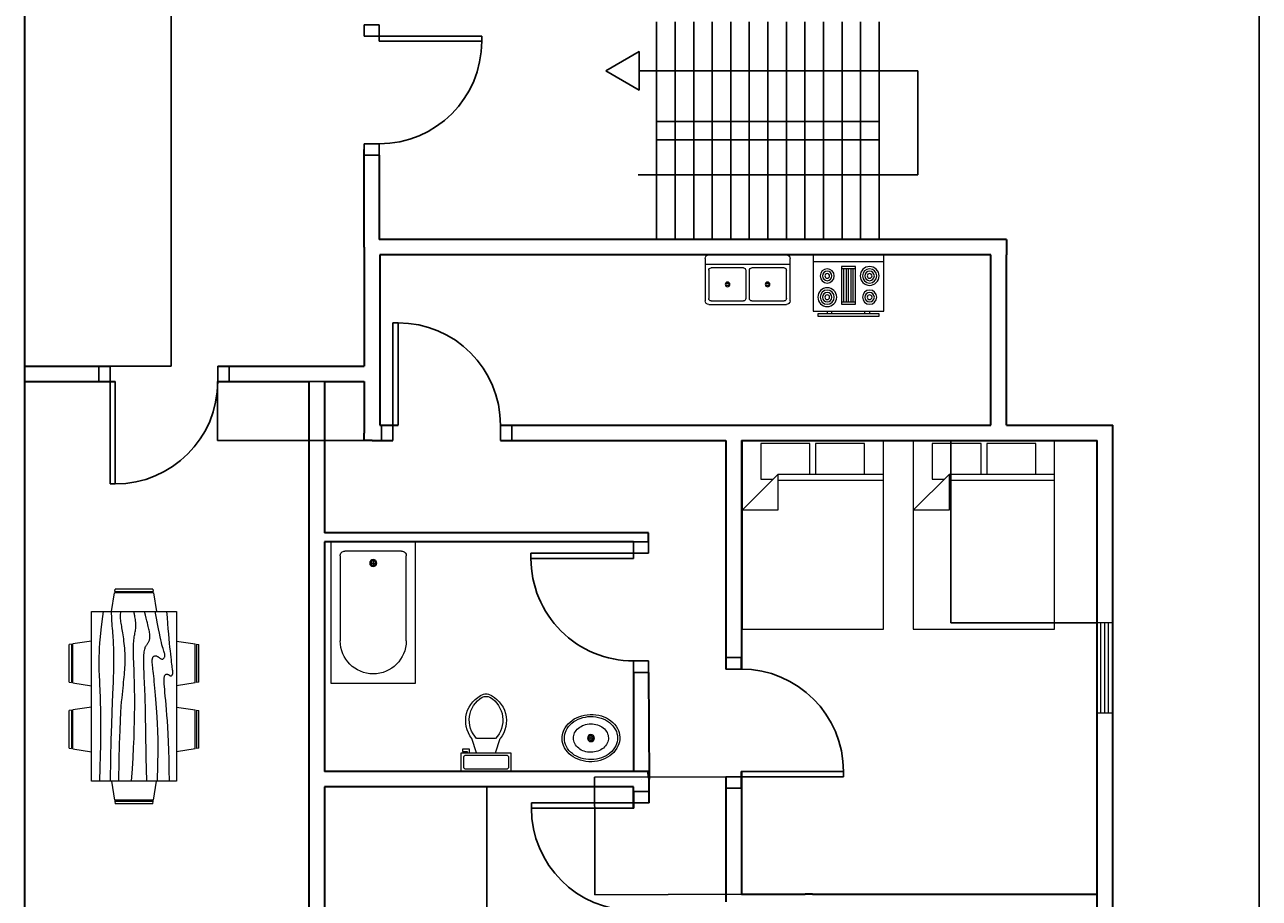
# Model space of a CAD drawing. Units: millimetres. Extents: x 31 to 27050, y -916 to 32407.
# Tile 4 of 7: x 13741 to 27050, y 7370 to 16782. Entities that reach past the tile are written whole.
import ezdxf

# ---------------------------------------------------------------- set-up
doc = ezdxf.new("R2010")
doc.units = ezdxf.units.MM
for name, color, linetype, lineweight in [('A-ANNO-DIMS', 2, 'Continuous', 18), ('A-DOOR', 3, 'Continuous', 25), ('A-EQPM', 8, 'Continuous', 18), ('A-FLOR-FIXT', 9, 'Continuous', 18), ('A-FLOR-STRS', 7, 'Continuous', 25), ('A-FURN', 8, 'Continuous', 13), ('A-GLAZ', 4, 'Continuous', 18), ('A-WALL', 7, 'Continuous', 35)]:
    doc.layers.add(name, color=color, linetype=linetype, lineweight=lineweight)
doc.styles.get("Standard").update_dxf_attribs({"font": 'arial.ttf'})
doc.dimstyles.get("Standard").update_dxf_attribs({"dimtxt": 0.18, "dimasz": 0.18, "dimexe": 0.18, "dimexo": 0.0625, "dimgap": 0.09, "dimtad": 0, "dimtih": 1, "dimtoh": 1, "dimdec": 4, "dimzin": 0, "dimdsep": 46, "dimtxsty": 'Standard', "dimcen": 0.09, "dimadec": 0, "dimazin": 0, "dimtfac": 1, "dimtdec": 4, "dimtofl": 0, "dimtmove": 0, "dimatfit": 3, "dimfxl": 1, "dimtolj": 1, "dimtzin": 0, "dimarcsym": 0})

# ---------------------------------------------------------------- blocks, each defined once
blk = doc.blocks.new('Bath Tub - 26 x 60 in.')
for p, q in [((8, -18), (10, -18)), ((9, -17), (9, -19))]:
    blk.add_line(p, q)
blk.add_lwpolyline([(0, -36), (0, 0), (60, 0), (60, -36)], close=True)
for points in [[(6, -4), (42, -4)], [(4, -30), (4, -6)], [(42, -32), (6, -32)]]:
    blk.add_lwpolyline(points)
for radius in [1.5, 1]:
    blk.add_circle((9, -18), radius)
for centre, radius, start, end in [((5.75, -5.75), 1.767766999999999, 81.86989999999999, 188.1301), ((42, -18), 14, 270, 90), ((5.75, -30.25), 1.767766999999999, 171.8699, 278.1301)]:
    blk.add_arc(centre, radius, start, end)
blk = doc.blocks.new('Sink - Oval top')
for p, q in [((-1, 0), (1, 0)), ((0, 1), (0, -1))]:
    blk.add_line(p, q)
for points in [[(-12.23371880354079, 0.3941914712607968, 0.1176342565883263), (-11.46456229543957, -3.361933235489118, 0.104469279667093), (-8.878748691070427, -6.803541973650567, 0.0900157896014849), (-5.082757700676665, -9.072309807490512, 0.0819199491592185), (-0.3227280122732736, -10.01585280257211, 0.0819199491592091), (4.488169920880977, -9.380701564817912, 0.0900157896014801), (8.422342359155778, -7.36101289847943, 0.1044692796670922), (11.22435122606941, -4.093009071543406, 0.1176342565883338), (12.23371880354091, -0.3941914712607968, 0.1176342565883057), (11.46456229543992, 3.361933235488777, 0.1044692796670849), (8.878748691070427, 6.803541973650567, 0.0900157896014884), (5.082757700676324, 9.072309807490681, 0.0819199491592058), (0.3227280122732736, 10.01585280257211, 0.081919949159207), (-4.488169920880864, 9.380701564817969, 0.0900157896014802), (-8.422342359155778, 7.36101289847943, 0.1044692796670951), (-11.22435122606919, 4.093009071543633, 0.1176342565883402)], [(-11.28627986850119, 0.1590597164737346, 0.1186217001864142), (-10.51590095791209, -3.253161772358112, 0.1046781721811095), (-8.071803350560115, -6.358618019863342, 0.0895620664691738), (-4.537699193222351, -8.366971929609804, 0.0811846988912177), (-0.1289739026695997, -9.15150355811437, 0.0811846988912276), (4.300109150126218, -8.491524865184601, 0.0895620664691798), (7.889406708212618, -6.583562428127606, 0.1046781721811044), (10.42004782883111, -3.548216131892445, 0.1186217001864013), (11.28627986850119, -0.1590597164736209, 0.1186217001863945), (10.51590095791221, 3.253161772357998, 0.1046781721811069), (8.071803350560115, 6.358618019863342, 0.0895620664691756), (4.537699193222124, 8.366971929609917, 0.081184698891216), (0.1289739026695997, 9.151503558114428, 0.0811846988912142), (-4.300109150125877, 8.491524865184829, 0.0895620664691747), (-7.889406708212618, 6.583562428127606, 0.1046781721811045), (-10.42004782883111, 3.548216131892445, 0.1186217001863946)], [(-7.420452389032902, 0.0829876781601797, 0.1182825673856775), (-6.907065465214486, -2.1674649380775, 0.1046074595377274), (-5.294791470712084, -4.209988192029413, 0.0897179636260996), (-2.966599981142508, -5.528122152688069, 0.0814360825277113), (-0.0675135187855176, -6.036810076758797, 0.0814360825277218), (2.84222437824053, -5.593085960977873, 0.0897179636261315), (5.199312936802016, -4.327350491993342, 0.1046074595376878), (6.85686365682659, -2.321395784920355, 0.1182825673856714), (7.420452389033016, -0.0829876781601797, 0.1182825673856961), (6.907065465214486, 2.167464938077614, 0.1046074595377135), (5.294791470712084, 4.209988192029413, 0.0897179636261265), (2.966599981142621, 5.528122152687842, 0.0814360825277426), (0.0675135187855176, 6.036810076758797, 0.0814360825277225), (-2.842224378240644, 5.593085960977873, 0.0897179636261212), (-5.199312936802016, 4.327350491993342, 0.1046074595377049), (-6.856863656826476, 2.321395784920355, 0.1182825673856712)]]:
    blk.add_lwpolyline(points, format="xyb", close=True)
for radius in [1.5, 1]:
    blk.add_circle((0, 0), radius)
blk = doc.blocks.new('Toilet - top')
for p, q in [((9.5, -6), (9.5, -2)), ((-10, -8.5), (-8, -8.5)), ((-10, -9.5), (-10, -8.5)), ((-7, -9.5), (-10, -9.5)), ((-8, -8.5), (-8, -8)), ((-7, -8), (-7, -9.5)), ((-4, -8), (-6, -14)), ((4, -8), (6, -14)), ((4, -14), (-4, -14))]:
    blk.add_line(p, q)
blk.add_lwpolyline([(10.5, -8), (10.5, 0), (-10.5, 0), (-10.5, -8)], close=True)
for points in [[(-9.5, -2), (-9.5, -6)], [(8.5, -1), (-8.5, -1)], [(-8.5, -7), (8.5, -7)]]:
    blk.add_lwpolyline(points)
for centre, radius, start, end in [((-8.625, -1.875), 0.8838834999999999, 81.86989999999999, 188.1301), ((8.625, -1.875), 0.8838834999999999, 351.8699, 98.13009999999998), ((-8.625, -6.125), 0.8838834999999999, 171.869898, 278.1301), ((8.625, -6.125), 0.8838834999999999, 261.8699, 8.130099999999993), ((3.519562435188956, -21.58049502388982), 12.16902005083646, 141.4691096810948, 247.9714346835576), ((4.199957580658807, -21.81740929088453), 11.3291791325804, 136.3677254423718, 238.946823937405), ((-3.519499936778316, -21.58047137067522), 12.16903423757823, 292.0284332733152, 38.53070636800453), ((-4.199890672038477, -21.81738596564128), 11.32918622148567, 301.0530065773863, 43.63209216694732), ((2.09660981727e-05, -27.87646475467881), 4, 245.7318247449371, 294.2681740488959), ((2.09415214183e-05, -28.99996806116075), 4, 254.8605283244437, 285.1394707718433)]:
    blk.add_arc(centre, radius, start, end)
blk = doc.blocks.new('Dining Set - 36 x 72 in.')
for p, q in [((-22, 27.5), (-22.15620000000001, 26.50042)), ((-5.841600000000028, 26.5), (-22.15340000000003, 26.5)), ((-22, 27.5), (-6, 27.5)), ((-5.843700000000012, 26.49966), (-6, 27.5)), ((6, 27.5), (5.843799999999987, 26.50042)), ((22.15839999999997, 26.5), (5.846599999999966, 26.5)), ((6, 27.5), (22, 27.5)), ((22.15629999999999, 26.49966), (22, 27.5)), ((-22.23430000000002, 26.00059), (-23.48470000000003, 17.99762)), ((-22.23040000000003, 26), (-5.760800000000017, 26)), ((-4.515199999999992, 17.99762), (-5.765500000000031, 25.99926)), ((5.765699999999981, 26.00059), (4.515299999999967, 17.99762)), ((5.769599999999968, 26), (22.23919999999998, 26)), ((23.48480000000001, 17.99762), (22.23449999999997, 25.99926)), ((36, 18), (-36, 18)), ((-36, 18), (-36, -18)), ((36, -18), (36, 18)), ((-45.49999999999999, 8.000000000000004), (-44.50040000000001, 8.156170000000007)), ((-45.49999999999999, 8.000000000000004), (-45.49999999999999, -7.999999999999996)), ((-44.5, -8.15843), (-44.5, 8.153380000000002)), ((-44.00060000000002, 8.234280000000002), (-35.99760000000003, 9.484740000000006)), ((-44, 8.230410000000003), (-44, -8.239149999999999)), ((44.00059999999996, 8.234280000000002), (35.99759999999998, 9.484740000000006)), ((44, 8.230410000000003), (44, -8.239149999999999)), ((44.5, -8.15843), (44.5, 8.153380000000002)), ((45.49999999999999, 8.000000000000004), (44.50049999999999, 8.156170000000007)), ((45.49999999999999, 8.000000000000004), (45.49999999999999, -7.999999999999996)), ((-44.49970000000002, -8.156309999999994), (-45.49999999999999, -7.999999999999996)), ((-35.99760000000003, -9.484759999999998), (-43.9993, -8.234499999999993)), ((35.99759999999998, -9.484759999999998), (43.9993, -8.234499999999993)), ((44.49969999999995, -8.156309999999994), (45.49999999999999, -7.999999999999996)), ((-36, -18), (36, -18)), ((-22.23430000000002, -26.0006), (-23.48470000000003, -17.99762)), ((-4.515199999999992, -17.99762), (-5.765500000000031, -25.99928)), ((5.765699999999981, -26.0006), (4.515299999999967, -17.99762)), ((23.48480000000001, -17.99762), (22.23449999999997, -25.99928)), ((-22.23040000000003, -26), (-5.760800000000017, -26)), ((5.769599999999968, -26), (22.23919999999998, -26)), ((-22, -27.5), (-22.15620000000001, -26.50044)), ((-5.841600000000028, -26.5), (-22.15340000000003, -26.5)), ((-22, -27.5), (-6, -27.5)), ((-5.843700000000012, -26.49967), (-6, -27.5)), ((6, -27.5), (5.843799999999987, -26.50044)), ((22.15839999999997, -26.5), (5.846599999999966, -26.5)), ((6, -27.5), (22, -27.5)), ((22.15629999999999, -26.49967), (22, -27.5))]:
    blk.add_line(p, q)
for points in [[(-36, 15), (-31.17720000000003, 14.97754), (-26.80790000000002, 14.91406), (-22.85380000000003, 14.81543), (-19.27600000000001, 14.6875), (-16.03620000000001, 14.53613), (-13.09570000000002, 14.36718), (-10.41590000000002, 14.18652), (-7.958300000000008, 14), (-5.690400000000011, 13.81315), (-3.603499999999996, 13.63021), (-1.695400000000006, 13.45508), (0.0364999999999896, 13.29166), (1.594499999999982, 13.14388), (2.981099999999969, 13.01562), (4.198800000000005, 12.9108), (5.25, 12.83333), (6.139299999999991, 12.78613), (6.880200000000002, 12.76823), (7.488299999999981, 12.77767), (7.979199999999991, 12.8125), (8.368499999999983, 12.87077), (8.671899999999994, 12.95052), (8.904899999999998, 13.0498), (9.083300000000008, 13.16666), (9.220499999999959, 13.29899000000001), (9.32159999999999, 13.44401), (9.389499999999998, 13.59879), (9.427099999999996, 13.76041), (9.437299999999993, 13.92594), (9.423200000000008, 14.09245), (9.387499999999989, 14.257), (9.333300000000008, 14.41666), (9.263800000000003, 14.56917), (9.183600000000013, 14.71484), (9.097499999999968, 14.85465), (9.010400000000004, 14.98958), (8.92719999999997, 15.12060000000001), (8.852899999999975, 15.2487), (8.79219999999998, 15.37483), (8.75, 15.5), (8.730500000000006, 15.62467), (8.734399999999994, 15.74739), (8.761699999999962, 15.86621), (8.8125, 15.97916), (8.886699999999962, 16.08431), (8.984399999999994, 16.17968), (9.105500000000006, 16.26334), (9.25, 16.33333), (9.418900000000008, 16.38802), (9.617199999999968, 16.42708), (9.850599999999986, 16.45052), (10.125, 16.45833), (10.44630000000001, 16.45052), (10.82029999999997, 16.42708), (11.25290000000001, 16.38802), (11.75, 16.33333), (12.3184, 16.26318), (12.96940000000001, 16.17838), (13.7151, 16.07991), (14.5677, 15.96875), (15.53949999999997, 15.84586), (16.64259999999996, 15.71224), (17.88929999999999, 15.56884), (19.29169999999999, 15.41666), (20.85899999999998, 15.25667), (22.58789999999999, 15.08984), (24.47210000000001, 14.91715), (26.5052, 14.73958), (28.68090000000001, 14.5581), (30.99289999999996, 14.3737), (33.43469999999996, 14.18733), (36, 14)], [(-36, 10), (-28.97660000000002, 10.14274000000001), (-23.17250000000001, 10.20442), (-18.42410000000001, 10.19775), (-14.5677, 10.13541), (-11.43990000000002, 10.03011), (-8.87700000000001, 9.894530000000007), (-6.715399999999988, 9.741370000000005), (-4.791699999999991, 9.58333), (-2.96980000000002, 9.43082), (-1.224600000000009, 9.285150000000005), (0.4414999999999623, 9.14534), (2.02600000000001, 9.010410000000004), (3.526599999999973, 8.879390000000004), (4.940799999999967, 8.751300000000004), (6.265999999999962, 8.625160000000005), (7.5, 8.500000000000004), (8.641099999999994, 8.375490000000003), (9.691399999999987, 8.253900000000005), (10.65379999999999, 8.13818), (11.53120000000001, 8.031250000000004), (12.32669999999996, 7.936030000000005), (13.043, 7.85547), (13.68309999999997, 7.792480000000001), (14.25, 7.750000000000003), (14.74709999999999, 7.730300000000003), (15.17969999999997, 7.733070000000001), (15.55369999999999, 7.757320000000003), (15.875, 7.80208), (16.14940000000001, 7.866370000000006), (16.38279999999997, 7.94922), (16.58109999999999, 8.04964), (16.75, 8.166660000000004), (16.89439999999996, 8.29915), (17.01429999999999, 8.445310000000003), (17.1089, 8.603190000000001), (17.17709999999999, 8.77083), (17.21799999999996, 8.946290000000001), (17.2305, 9.127600000000005), (17.21369999999996, 9.312820000000006), (17.16669999999999, 9.500000000000004), (17.08949999999999, 9.687500000000004), (16.98699999999996, 9.875000000000004), (16.86489999999998, 10.0625), (16.72919999999999, 10.25), (16.5856, 10.4375), (16.44009999999997, 10.625), (16.29849999999999, 10.8125), (16.16669999999999, 11), (16.05000000000001, 11.18733), (15.95179999999999, 11.3737), (15.8752, 11.5581), (15.8229, 11.73958), (15.798, 11.91715), (15.80340000000001, 12.08984), (15.84199999999998, 12.25667), (15.91669999999999, 12.41666), (16.02949999999998, 12.56836), (16.17840000000001, 12.70833), (16.3605, 12.83268), (16.5729, 12.9375), (16.8127, 13.01888000000001), (17.07679999999999, 13.07291), (17.36250000000001, 13.0957), (17.66669999999999, 13.08333), (17.98939999999999, 13.03312), (18.34179999999998, 12.94726), (18.7382, 12.82918), (19.1927, 12.68229), (19.71949999999998, 12.51001), (20.33269999999999, 12.31575), (21.04649999999998, 12.10294), (21.875, 11.875), (22.83569999999997, 11.63354), (23.95900000000001, 11.37304), (25.27859999999999, 11.08618), (26.82819999999998, 10.76562), (28.64139999999998, 10.40405), (30.75200000000001, 9.994140000000005), (33.1936, 9.528560000000002), (36, 9.000000000000004)], [(-36, 5.500000000000003), (-30.71570000000003, 5.334800000000004), (-26.06900000000002, 5.20963), (-21.99459999999999, 5.11767), (-18.42709999999999, 5.05208), (-15.30090000000001, 5.006020000000003), (-12.55080000000004, 4.972650000000005), (-10.1112, 4.945150000000001), (-7.916699999999991, 4.916660000000003), (-5.908999999999991, 4.881670000000003), (-4.058600000000012, 4.839840000000005), (-2.342899999999985, 4.792150000000003), (-0.7395999999999959, 4.73958), (0.7738999999999692, 4.683100000000006), (2.21999999999997, 4.623700000000003), (3.621299999999962, 4.562330000000006), (5, 4.500000000000003), (6.37299999999999, 4.437820000000005), (7.734399999999993, 4.377600000000004), (9.072299999999984, 4.321290000000001), (10.375, 4.27083), (11.63089999999999, 4.228190000000001), (12.8281, 4.195310000000002), (13.95509999999996, 4.17415), (15, 4.166660000000003), (15.95400000000001, 4.174480000000006), (16.81899999999996, 4.197910000000003), (17.6001, 4.236980000000006), (18.30209999999999, 4.291660000000003), (18.92989999999997, 4.361980000000006), (19.48829999999998, 4.447910000000003), (19.98230000000001, 4.549480000000006), (20.41669999999999, 4.666660000000003), (20.79689999999999, 4.798990000000006), (21.1302, 4.944010000000002), (21.42449999999997, 5.098790000000004), (21.6875, 5.260410000000003), (21.92709999999999, 5.42594), (22.15109999999999, 5.592450000000003), (22.36719999999997, 5.757000000000001), (22.58339999999998, 5.916660000000003), (22.80649999999997, 6.068680000000004), (23.04039999999998, 6.210930000000001), (23.28789999999998, 6.341470000000004), (23.5521, 6.45833), (23.83580000000001, 6.559570000000004), (24.142, 6.643230000000006), (24.4735, 6.707350000000001), (24.83339999999998, 6.750000000000003), (25.2235, 6.76969), (25.642, 6.766920000000002), (26.08580000000001, 6.74267), (26.5521, 6.697910000000003), (27.03789999999998, 6.633620000000004), (27.54039999999998, 6.550780000000006), (28.05649999999997, 6.450360000000006), (28.58339999999998, 6.33333), (29.12419999999997, 6.19987), (29.70709999999997, 6.046870000000001), (30.36609999999996, 5.870440000000005), (31.1354, 5.666660000000003), (32.04929999999996, 5.431640000000005), (33.142, 5.161460000000001), (34.44749999999999, 4.852210000000003), (36, 4.500000000000003)], [(-36, -0.9999999999999964), (-30.79150000000004, -0.6590999999999987), (-26.01949999999999, -0.3821599999999954), (-21.65190000000001, -0.1628399999999992), (-17.65629999999999, 0.0052100000000017), (-14.00049999999999, 0.1283300000000018), (-10.65230000000002, 0.2128900000000051), (-7.579600000000027, 0.2652200000000029), (-4.75, 0.2916600000000038), (-2.134000000000014, 0.2979300000000045), (0.2878000000000043, 0.287110000000002), (2.5317, 0.2616300000000002), (4.614599999999995, 0.2239600000000017), (6.552899999999965, 0.1765100000000039), (8.363299999999981, 0.1217400000000062), (10.06229999999999, 0.0620900000000013), (11.66669999999999, 3.6e-15), (13.18989999999996, -0.0620099999999972), (14.63409999999999, -0.1210999999999949), (15.9982, -0.174319999999998), (17.28129999999999, -0.2187499999999964), (18.48230000000001, -0.2514699999999941), (19.6003, -0.2695299999999996), (20.6343, -0.2700199999999988), (21.58339999999999, -0.2499999999999964), (22.44810000000001, -0.2076799999999999), (23.23570000000001, -0.1458399999999962), (23.95490000000001, -0.0683599999999949), (24.6146, 0.0208300000000001), (25.2235, 0.1178400000000046), (25.79039999999998, 0.2187500000000035), (26.32409999999999, 0.3196600000000025), (26.83339999999998, 0.4166600000000038), (27.32650000000001, 0.5061800000000041), (27.80989999999997, 0.5859300000000012), (28.2894, 0.6539700000000046), (28.77089999999999, 0.7083300000000002), (29.26009999999997, 0.7470700000000045), (29.76299999999998, 0.7682300000000062), (30.28550000000001, 0.7698500000000017), (30.83339999999998, 0.7500000000000036), (31.40879999999999, 0.707840000000001), (31.99939999999998, 0.6471300000000006), (32.589, 0.5727500000000028), (33.16149999999999, 0.4895800000000002), (33.70079999999996, 0.402500000000007), (34.19079999999997, 0.3164000000000051), (34.61529999999999, 0.2361600000000017), (34.95839999999998, 0.1666600000000038), (35.20990000000001, 0.1116500000000009), (35.38479999999998, 0.0703100000000028), (35.50399999999996, 0.0406900000000015), (35.58859999999999, 0.0208300000000001), (35.65940000000001, 0.0087900000000012), (35.73769999999996, 0.0026000000000046), (35.8442, 0.0003200000000056), (36, 3.6e-15)], [(-36, -6.499999999999996), (-27.18430000000001, -6.312669999999993), (-20.084, -6.126299999999996), (-14.46899999999999, -5.941899999999993), (-10.10939999999999, -5.760419999999999), (-6.77520000000004, -5.582849999999996), (-4.236300000000028, -5.410159999999994), (-2.262900000000001, -5.243329999999996), (-0.625, -5.083339999999996), (0.8707999999999742, -4.930989999999997), (2.271500000000003, -4.786459999999994), (3.587199999999995, -4.649739999999997), (4.828100000000006, -4.520839999999996), (6.004599999999982, -4.399739999999997), (7.127000000000009, -4.286459999999994), (8.205299999999966, -4.180989999999997), (9.25, -4.083339999999996), (10.27049999999997, -3.993819999999995), (11.27339999999998, -3.914069999999998), (12.2647, -3.846029999999995), (13.25, -3.791669999999999), (14.23539999999997, -3.752929999999995), (15.22659999999996, -3.731769999999993), (16.22949999999997, -3.730149999999998), (17.25, -3.749999999999996), (18.2912, -3.792479999999994), (19.3451, -3.855469999999993), (20.40089999999998, -3.936039999999994), (21.4479, -4.031249999999996), (22.47539999999998, -4.138189999999998), (23.47269999999998, -4.253909999999994), (24.4289, -4.375489999999995), (25.33339999999999, -4.499999999999996), (26.17849999999999, -4.624919999999999), (26.96940000000001, -4.749349999999996), (27.71449999999999, -4.872809999999997), (28.4219, -4.994789999999998), (29.09999999999996, -5.114829999999994), (29.75720000000001, -5.232419999999994), (30.40159999999997, -5.347089999999997), (31.04169999999999, -5.458339999999996), (31.68369999999999, -5.564369999999993), (32.32619999999997, -5.658209999999993), (32.9658, -5.731529999999995), (33.59899999999999, -5.776039999999998), (34.22239999999999, -5.783449999999998), (34.83269999999999, -5.745449999999994), (35.4264, -5.653729999999999), (36, -5.499999999999996)], [(-36, -9.999999999999996), (-26.40219999999999, -9.812989999999996), (-18.46750000000003, -9.628909999999994), (-11.9839, -9.450689999999998), (-6.739599999999995, -9.281249999999996), (-2.522600000000011, -9.123539999999995), (0.8788999999999872, -8.980469999999993), (3.676899999999989, -8.854979999999994), (6.083300000000008, -8.749999999999996), (8.276700000000005, -8.667649999999998), (10.30209999999999, -8.606769999999994), (12.1712, -8.565429999999996), (13.89580000000001, -8.54167), (15.48759999999998, -8.533529999999995), (16.95830000000001, -8.539069999999999), (18.31970000000001, -8.556319999999994), (19.58339999999998, -8.583339999999996), (20.76159999999999, -8.618409999999994), (21.86849999999998, -8.660809999999994), (22.91879999999998, -8.710039999999996), (23.9271, -8.765629999999998), (24.90809999999999, -8.827069999999996), (25.87629999999996, -8.89388), (26.84649999999999, -8.96558), (27.83339999999999, -9.04167), (28.84739999999999, -9.121179999999997), (29.88279999999998, -9.201169999999994), (30.93000000000001, -9.278239999999993), (31.97919999999999, -9.348959999999995), (33.02049999999997, -9.409909999999998), (34.04429999999996, -9.45768), (35.04069999999996, -9.488849999999996), (36, -9.499999999999996)], [(-36, -14.5), (-30.0881, -14.33512999999999), (-25.03320000000002, -14.21224), (-20.7312, -14.12646999999999), (-17.0781, -14.07292), (-13.97000000000003, -14.04670999999999), (-11.30270000000001, -14.04296999999999), (-8.972399999999993, -14.05680999999999), (-6.875, -14.08333999999999), (-4.922400000000038, -14.11832999999999), (-3.09050000000002, -14.16015999999999), (-1.370900000000006, -14.20784999999999), (0.2447999999999979, -14.26042), (1.764700000000004, -14.31689999999999), (3.197299999999984, -14.37629999999999), (4.550700000000006, -14.43766999999999), (5.833300000000008, -14.5), (7.055399999999963, -14.5621), (8.235000000000014, -14.62174999999999), (9.392200000000003, -14.67652), (10.54689999999999, -14.72395999999999), (11.7192, -14.76164), (12.92899999999997, -14.78711), (14.19649999999996, -14.79794), (15.54169999999999, -14.79167), (16.99329999999998, -14.76423999999999), (18.61519999999996, -14.70508), (20.48039999999998, -14.60197), (22.66149999999999, -14.44270999999999), (25.2312, -14.21509), (28.26240000000002, -13.90689999999999), (31.8277, -13.50594), (36, -13)]]:
    blk.add_lwpolyline(points)
blk = doc.blocks.new('Range-Oven - 30 in top')
for p, q in [((0, -3), (30, -3)), ((12, -6), (18, -6)), ((13, -19.999996), (13, -6)), ((14, -6), (14, -19.999996)), ((15, -19.999996), (15, -6)), ((16, -6), (16, -19.999996)), ((17, -19.999996), (17, -6)), ((18, -19.999996), (12, -19.999996)), ((6.000000000000003, -23.99999600000001), (6.000000000000003, -24.999996)), ((8.000000000000004, -24.999996), (8.000000000000004, -23.99999600000001)), ((22.00000000000001, -24.999996), (22.00000000000001, -23.99999600000001)), ((24, -23.99999600000001), (24, -24.999996))]:
    blk.add_line(p, q)
for points in [[(0, -23.99999600000001), (0, 0), (30, 0), (30, -23.99999600000001)], [(12, -20.999996), (12, -5), (18, -5), (18, -20.999996)], [(2.000000000000003, -25.999996), (2.000000000000003, -24.999996), (28.00000000000001, -24.999996), (28.00000000000001, -25.999996)]]:
    blk.add_lwpolyline(points, close=True)
for centre, radius in [((6.000000000000003, -9.0000002), 4), ((6.000000000000003, -9.0000002), 3), ((6.000000000000003, -9.0000002), 2), ((6.000000000000003, -9.0000002), 1), ((24, -9.0000002), 3), ((24, -9.0000002), 2), ((24, -9.0000002), 1), ((6.000000000000003, -18), 3), ((24, -18), 4), ((24, -18), 3), ((6.000000000000003, -18), 2), ((6.000000000000003, -18), 1), ((24, -18), 2), ((24, -18), 1)]:
    blk.add_circle(centre, radius)
blk = doc.blocks.new('Sink-double - 36 in top')
for p, q in [((-18, -4), (18, -4)), ((-0.75, -18.5), (-0.75, -6.5)), ((0.75, -6.5), (0.75, -18.5))]:
    blk.add_line(p, q)
for points in [[(-16.5, 0), (16.5, 0)], [(-18, -19.5), (-18, -1.5)], [(18, -1.5), (18, -19.5)], [(-16.5, -18.5), (-16.5, -6.5)], [(-15.5, -5.5), (-1.75, -5.5)], [(1.75, -5.5), (15.5, -5.5)], [(16.5, -6.5), (16.5, -18.5)], [(-1.75, -19.5), (-15.5, -19.5)], [(15.5, -19.5), (1.75, -19.5)], [(16.5, -21), (-16.5, -21)]]:
    blk.add_lwpolyline(points)
for centre, radius in [((-8.5, -12.5), 1), ((-8.5, -12.5), 0.5), ((8.5, -12.5), 1), ((8.5, -12.5), 0.5)]:
    blk.add_circle(centre, radius)
for centre, radius, start, end in [((-16.5, -1.5), 1.5, 90, 180), ((16.5, -1.5), 1.5, 0, 90), ((-15.5, -6.5), 1, 90, 180), ((-1.75, -6.5), 1, 0, 90), ((1.75, -6.5), 1, 90, 180), ((15.5, -6.5), 1, 0, 90), ((-16.5, -19.5), 1.5, 180, 270), ((-15.5, -18.5), 1, 180, 270), ((-1.75, -18.5), 1, 270, 0), ((1.75, -18.5), 1, 180, 270), ((15.5, -18.5), 1, 270, 0), ((16.5, -19.5), 1.5, 270, 0)]:
    blk.add_arc(centre, radius, start, end)
blk = doc.blocks.new('Bed - Queen')
for p, q in [((0, -80.00003000000002), (0, 0)), ((0, 0), (59.99998999999999, 0)), ((59.99998999999999, 0), (59.99998999999999, -80.00003000000002)), ((7.99999, -1.200000000000017), (28.79998, -1.200000000000017)), ((7.99999, -14.4), (7.99999, -1.200000000000017)), ((28.79998, -1.200000000000017), (28.79998, -14.4)), ((31.19999, -1.200000000000017), (51.99999000000001, -1.200000000000017)), ((31.19999, -14.4), (31.19999, -1.200000000000017)), ((51.99999000000001, -1.200000000000017), (51.99999000000001, -16.4)), ((0, -14.4), (44.79999999999999, -14.4)), ((59.99998999999999, -29.60000000000001), (44.79999999999999, -14.4)), ((44.79999999999999, -14.4), (44.79999999999999, -29.60000000000001)), ((44.79999999999999, -16.80000000000001), (0, -16.80000000000001)), ((51.99999000000001, -16.4), (46.79936, -16.4)), ((44.79999999999999, -29.60000000000001), (59.99998999999999, -29.60000000000001)), ((59.99998999999999, -80.00003000000002), (0, -80.00003000000002))]:
    blk.add_line(p, q)
blk = doc.blocks.new('Window - Wood Frame 36 in. Wide plan')
for p, q in [((0, 6), (0, 0)), ((36, 6), (36, 0)), ((0, 4.5), (36, 4.5)), ((0, 3), (36, 3)), ((0, 1.5), (36, 1.5))]:
    blk.add_line(p, q)
blk = doc.blocks.new('DOOR-SINGLE-1104')
for p, q in [((56.41678681898429, 1104.337341461596), (-7.18501e-11, 1104.337341461596)), ((-7.18501e-11, 1104.337341461596), (-7.18501e-11, 3.638e-12)), ((56.41678681898429, 7.276e-12), (56.41678681898429, 1104.337341461596)), ((-1226.913698425656, -163.8831223050438), (-1226.913698425656, 3.638e-12)), ((-1104.337341461589, 3.638e-12), (-1226.913698425656, 7.276e-12)), ((-1104.337341461589, 3.638e-12), (-1104.337341461589, -163.8831223050438)), ((-7.18501e-11, 3.638e-12), (56.41678681898429, 7.276e-12)), ((56.41678681898429, -163.8831223050438), (56.41678681898429, 3.638e-12)), ((56.41678681898429, 3.638e-12), (178.9931437830519, 3.638e-12)), ((178.9931437830519, 3.638e-12), (178.9931437830519, -163.8831223050438)), ((-1104.337341461589, -163.8831223050438), (-1226.913698425656, -163.8831223050438)), ((178.9931437830519, -163.8831223050438), (56.41678681898429, -163.8831223050438))]:
    blk.add_line(p, q)
blk.add_arc((0, 3.638e-12), 1104.337341461589, 90, 180)
blk = doc.blocks.new('STAIR-RETURN-2400')
for p, q in [((9.095e-13, 2345.636859649549), (9.095e-13, -1.819e-12)), ((200.0000000000009, 2345.636859649549), (200.0000000000009, -1.819e-12)), ((400.0000000000008, 2345.636859649549), (400.0000000000008, -1.819e-12)), ((600.0000000000008, 2345.636859649549), (600.0000000000008, -1.819e-12)), ((800.0000000000008, 2345.636859649552), (800.0000000000008, 1.819e-12)), ((1000.000000000001, 2345.636859649556), (1000.000000000001, 5.457e-12)), ((1200.000000000001, 2345.636859649556), (1200.000000000001, 5.457e-12)), ((1400.000000000001, 2345.636859649556), (1400.000000000001, 5.457e-12)), ((1600.000000000001, 2345.636859649559), (1600.000000000001, 9.0949e-12)), ((1800.000000000001, 2345.636859649559), (1800.000000000001, 9.0949e-12)), ((2000.000000000001, 2345.636859649559), (2000.000000000001, 9.0949e-12)), ((2200.000000000001, 2345.636859649563), (2200.000000000001, 1.27329e-11)), ((2400.000000000001, 2345.636859649563), (2400.000000000001, 1.27329e-11)), ((-415.9249645337103, 697.4958917418807), (-415.9249645337103, 1817.654410237617)), ((-415.9249645337103, 1817.654410237617), (2588.331988211024, 1817.654410237617)), ((9.095e-13, 1172.818429824772), (9.095e-13, 1272.818429824772)), ((9.095e-13, 1272.818429824772), (2400.000000000001, 1272.818429824774)), ((2400.000000000001, 1272.818429824774), (2400.000000000001, 1072.818429824774)), ((2400.000000000001, 1072.818429824774), (9.095e-13, 1072.818429824774)), ((2597.09055342863, 697.4958917418807), (-415.9249645337103, 697.4958917418807))]:
    blk.add_line(p, q)
blk.add_lwpolyline([(2948.607295106225, 1817.654410237617), (2588.331988211024, 2025.65945565594), (2588.331988211024, 1609.649364819299)], close=True)
blk = doc.blocks.new('*D47')
at = {"layer": 'A-ANNO-DIMS', "color": 0, "lineweight": -2, "transparency": 16777216}
for p, q in [((25471.21116800002, 30827.53125900001), (27050.32866800003, 30827.53125900001)), ((27050.14866800003, 30827.35125900001), (27050.14866800003, 15745.77166202933)), ((27050.14866800004, 663.8281360000004), (27050.14866800003, 15745.40773297067)), ((25471.21116800002, 663.6481360000002), (27050.32866800003, 663.6481360000004))]:
    blk.add_line(p, q, dxfattribs=at)
at = {"layer": 'A-ANNO-DIMS', "color": 0, "transparency": 16777216}
for points in [[(27050.11866800003, 30827.35125900001), (27050.17866800003, 30827.35125900001), (27050.14866800003, 30827.53125900001)], [(27050.11866800004, 663.8281360000004), (27050.17866800004, 663.8281360000004), (27050.14866800004, 663.6481360000004)]]:
    blk.add_solid(points, dxfattribs=at)
at = {"layer": 'Defpoints', "color": 0, "transparency": 16777216}
for p in [(25471.14866800002, 30827.53125900001), (27050.14866800003, 30827.53125900001), (25471.14866800002, 663.6481360000002)]:
    blk.add_point(p, dxfattribs=at)
at = {"layer": 'A-ANNO-DIMS', "color": 0, "transparency": 16777216, "insert": (27050.14866800003, 15745.58969749999), "char_height": 0.18, "attachment_point": 5}
blk.add_mtext('\\A1;30164', dxfattribs=at)
blk = doc.blocks.new('*D65')
at = {"layer": 'A-ANNO-DIMS', "color": 0, "lineweight": -2, "transparency": 16777216}
for p, q in [((20302.73551700001, 8571.211099000004), (18723.61801700001, 8571.211099000004)), ((18723.79801700001, 8571.031099000003), (18723.79801700001, 4699.551179000002)), ((18723.79801700001, 827.7112590000002), (18723.79801700001, 4699.191179000002)), ((20302.73551700001, 827.5312590000003), (18723.61801700001, 827.5312590000002))]:
    blk.add_line(p, q, dxfattribs=at)
at = {"layer": 'A-ANNO-DIMS', "color": 0, "transparency": 16777216}
for points in [[(18723.76801700001, 8571.031099000003), (18723.82801700001, 8571.031099000003), (18723.79801700001, 8571.211099000004)], [(18723.76801700001, 827.7112590000002), (18723.82801700001, 827.7112590000002), (18723.79801700001, 827.5312590000002)]]:
    blk.add_solid(points, dxfattribs=at)
at = {"layer": 'Defpoints', "color": 0, "transparency": 16777216}
for p in [(18723.79801700001, 8571.211099000004), (20302.79801700001, 8571.211099000004), (20302.79801700001, 827.5312590000003)]:
    blk.add_point(p, dxfattribs=at)
at = {"layer": 'A-ANNO-DIMS', "color": 0, "transparency": 16777216, "insert": (18723.79801700001, 4699.371178999996), "char_height": 0.18, "attachment_point": 5}
blk.add_mtext('\\A1;7744', dxfattribs=at)
blk = doc.blocks.new('*D67')
at = {"layer": 'A-ANNO-DIMS', "color": 0, "lineweight": -2, "transparency": 16777216}
for p, q in [((13740.64783300001, 17938.12750700001), (15319.76533300001, 17938.12750700001)), ((15319.58533300001, 17937.94750700001), (15319.58533300001, 15520.25103252934)), ((15319.58533300001, 13102.19062900001), (15319.58533300001, 15519.88710347067)), ((13740.64783300001, 13102.01062900001), (15319.76533300001, 13102.01062900001))]:
    blk.add_line(p, q, dxfattribs=at)
at = {"layer": 'A-ANNO-DIMS', "color": 0, "transparency": 16777216}
for points in [[(15319.55533300001, 17937.94750700001), (15319.61533300001, 17937.94750700001), (15319.58533300001, 17938.12750700001)], [(15319.55533300001, 13102.19062900001), (15319.61533300001, 13102.19062900001), (15319.58533300001, 13102.01062900001)]]:
    blk.add_solid(points, dxfattribs=at)
at = {"layer": 'Defpoints', "color": 0, "transparency": 16777216}
for p in [(13740.58533300001, 17938.12750700001), (13740.58533300001, 13102.01062900001), (15319.58533300001, 13102.01062900001)]:
    blk.add_point(p, dxfattribs=at)
at = {"layer": 'A-ANNO-DIMS', "color": 0, "transparency": 16777216, "insert": (15319.58533300002, 15520.069068), "char_height": 0.18, "attachment_point": 5}
blk.add_mtext('\\A1;4836', dxfattribs=at)
blk = doc.blocks.new('*D72')
at = {"layer": 'A-ANNO-DIMS', "color": 0, "lineweight": -2, "transparency": 16777216}
for p, q in [((17399.426108, 12938.12750700001), (15820.30860800001, 12938.12750700001)), ((15820.48860800001, 12937.947507), (15820.48860800001, 12620.17599252934)), ((15820.48860800001, 12302.04054900001), (15820.48860800001, 12619.81206347068)), ((17399.426108, 12301.860549), (15820.30860800001, 12301.860549))]:
    blk.add_line(p, q, dxfattribs=at)
at = {"layer": 'A-ANNO-DIMS', "color": 0, "transparency": 16777216}
for points in [[(15820.45860800001, 12937.947507), (15820.51860800001, 12937.947507), (15820.48860800001, 12938.12750700001)], [(15820.45860800001, 12302.04054900001), (15820.51860800001, 12302.04054900001), (15820.48860800001, 12301.860549)]]:
    blk.add_solid(points, dxfattribs=at)
at = {"layer": 'Defpoints', "color": 0, "transparency": 16777216}
for p in [(15820.48860800001, 12938.12750700001), (17399.48860800001, 12938.12750700001), (17399.48860800001, 12301.860549)]:
    blk.add_point(p, dxfattribs=at)
at = {"layer": 'A-ANNO-DIMS', "color": 0, "transparency": 16777216, "insert": (15820.48860800001, 12619.994028), "char_height": 0.18, "attachment_point": 5}
blk.add_mtext('\\A1;636.3', dxfattribs=at)
blk = doc.blocks.new('*D82')
at = {"layer": 'A-ANNO-DIMS', "color": 0, "lineweight": -2, "transparency": 16777216}
for p, q in [((25302.73551700001, 12301.860549), (23723.61801700002, 12301.860549)), ((23723.79801700001, 12301.68054900001), (23723.79801700001, 11320.78903663779)), ((23723.79801700001, 10339.533718), (23723.79801700001, 11320.42523036221)), ((25302.73551700001, 10339.353718), (23723.61801700002, 10339.353718))]:
    blk.add_line(p, q, dxfattribs=at)
at = {"layer": 'A-ANNO-DIMS', "color": 0, "transparency": 16777216}
for points in [[(23723.76801700002, 12301.68054900001), (23723.82801700001, 12301.68054900001), (23723.79801700001, 12301.860549)], [(23723.76801700002, 10339.533718), (23723.82801700001, 10339.533718), (23723.79801700001, 10339.353718)]]:
    blk.add_solid(points, dxfattribs=at)
at = {"layer": 'Defpoints', "color": 0, "transparency": 16777216}
for p in [(23723.79801700001, 12301.860549), (25302.79801700002, 12301.860549), (25302.79801700002, 10339.353718)]:
    blk.add_point(p, dxfattribs=at)
at = {"layer": 'A-ANNO-DIMS', "color": 0, "transparency": 16777216, "insert": (23723.79801700001, 11320.60713349999), "char_height": 0.18, "attachment_point": 5}
blk.add_mtext('\\A1;1962.5', dxfattribs=at)
blk = doc.blocks.new('*D91')
at = {"layer": 'A-ANNO-DIMS', "color": 0, "lineweight": -2, "transparency": 16777216}
for p, q in [((21463.2836123898, 8679.383256266126), (19884.1759599213, 8673.806220645713)), ((19884.35659451226, 8673.626857481862), (19886.58908056331, 8041.510434497784)), ((19888.82285149227, 7409.030205238119), (19886.59036544123, 8041.146628222202)), ((21467.75114038979, 7414.426606266125), (19888.64348832843, 7408.849570647148))]:
    blk.add_line(p, q, dxfattribs=at)
at = {"layer": 'A-ANNO-DIMS', "color": 0, "transparency": 16777216}
for points in [[(19884.38659432516, 8673.626963434124), (19884.32659469936, 8673.6267515296), (19884.3559587987, 8673.806856359271)], [(19888.85285130517, 7409.030311190379), (19888.79285167937, 7409.030099285859), (19888.82348720583, 7408.85020636071)]]:
    blk.add_solid(points, dxfattribs=at)
at = {"layer": 'Defpoints', "color": 0, "transparency": 16777216}
for p in [(19884.3559587987, 8673.806856359271), (21463.34611200001, 8679.383477000001), (21467.81364000001, 7414.426827000001)]:
    blk.add_point(p, dxfattribs=at)
at = {"layer": 'A-ANNO-DIMS', "color": 0, "transparency": 16777216, "insert": (19886.58972300226, 8041.328531359996), "char_height": 0.18, "attachment_point": 5}
blk.add_mtext('\\A1;1265', dxfattribs=at)

msp = doc.modelspace()

# ---------------------------------------------------------------- linework, layer by layer
at = {"layer": 'A-DOOR'}
for p, q in [((20303.06755308104, 11210.33651640691), (20466.95067538609, 11210.33651640691)), ((20307.26554580139, 8521.175884980112), (20471.14866810643, 8521.175884980112)), ((21463.34611150464, 8556.807120053505), (21299.46298919959, 8556.807120053505))]:
    msp.add_line(p, q, dxfattribs=at)
at = {"layer": 'A-WALL'}
for p, q in [((13740.58533261045, 13102.01062910059), (13740.58533261045, 17938.12750679554)), ((17399.48860787868, 14467.4249367068), (17399.48860787868, 15437.28495533102)), ((17563.37173018373, 15375.99677684899), (17563.37173018373, 14467.4249367068)), ((17399.48860787868, 14384.27405581066), (17399.48860787868, 14467.4249367068)), ((17399.48860787868, 14384.27405581066), (17399.48860787868, 13102.01062910059)), ((24323.82982953254, 14467.4249367068), (17563.37173018373, 14467.4249367068)), ((24323.82982953254, 14467.4249367068), (24323.82982953254, 14303.54181440175)), ((24155.47917882185, 14303.54181440175), (17567.83925858937, 14303.54181440175)), ((17567.83925858937, 14303.54181440175), (17567.83925858937, 12465.74367114626)), ((24155.47917882185, 12465.74367114627), (24155.47917882185, 14303.54181440175)), ((24323.82982953254, 12465.74367114627), (24323.82982953254, 14303.54181440175)), ((13740.58533261045, 13102.01062910059), (14660.83659543506, 13102.01062910059)), ((13740.58533261045, 12938.12750679554), (13740.58533261045, 13102.01062910059)), ((15821.59072371564, 13102.01062910059), (17399.48860787868, 13102.01062910059)), ((13740.58533261045, 827.5312586717337), (13740.58533261045, 12938.12750679554)), ((13740.58533261045, 12938.12750679554), (14717.25338225412, 12938.12750679554)), ((15821.59072371564, 12938.12750679554), (16802.79801739574, 12938.12750679554)), ((16802.79801739574, 12938.12750679554), (16802.79801739574, 827.5312586717337)), ((16971.14866810643, 12938.12750679554), (17399.48860787868, 12938.12750679554)), ((16971.14866810643, 12938.12750679554), (16971.14866810643, 11309.00881926711)), ((17399.48860787868, 12938.12750679554), (17399.48860787868, 12382.59279025013)), ((17399.48860787868, 12301.86054884122), (17399.48860787868, 12382.59279025013)), ((17567.83925858937, 12465.74367114626), (17765.74253504597, 12465.74367114626)), ((18870.07987650749, 12465.74367114626), (24155.47917882185, 12465.74367114627)), ((24323.82982953254, 12465.74367114627), (25302.79801739574, 12465.74367114627)), ((25302.79801739574, 12465.74367114627), (25471.14866810643, 12465.74367114627)), ((25471.14866810643, 744.3803777755929), (25471.14866810643, 12465.74367114627)), ((17487.27592309339, 12301.86054884122), (17399.48860787868, 12301.86054884122)), ((17487.27592309339, 12301.86054884122), (17709.32574822692, 12301.86054884122)), ((18870.07987650749, 12301.86054884122), (21299.46298919959, 12301.86054884121)), ((21299.46298919959, 12301.86054884122), (21299.46298919959, 9840.137605298149)), ((21467.81363991029, 12301.86054884122), (25302.79801739574, 12301.86054884122)), ((21467.81363991029, 12301.86054884122), (21467.81363991029, 9840.128568706263)), ((25302.79801739574, 5827.531258671735), (25302.79801739574, 12301.86054884122)), ((20466.95067538609, 11309.00881926711), (16971.14866810643, 11309.00881926711)), ((16971.14866810643, 11210.33651640691), (16971.14866810643, 8735.094220936826)), ((20303.06755308104, 11210.33651640691), (16971.14866810643, 11210.33651640691)), ((20466.95067538609, 11210.33651640691), (20466.95067538609, 11309.00881926711)), ((20303.06755308103, 9804.429674198203), (20303.06755308103, 8735.094220936826)), ((20466.95067538608, 9804.429674198203), (20471.14866810643, 8651.943340040685)), ((20390.58533261046, 8735.094220936826), (16971.14866810643, 8735.094220936826)), ((20471.14866810643, 8735.094220936828), (20390.58533261046, 8735.094220936826)), ((20390.58533261046, 8651.943340040685), (20390.58533261046, 8651.943340040685)), ((20471.14866810643, 8651.943340040685), (20459.02176268279, 8735.094220936828)), ((20471.14866810643, 8651.943340040685), (20471.14866810643, 8735.094220936828)), ((20471.14866810643, 8398.599528016042), (20471.14866810643, 8651.943340040685)), ((21299.46298919959, 8679.383477017574), (21299.46298919959, 7331.275946538546)), ((21467.81363991029, 8735.80026383663), (21467.81363991029, 7414.426827434685)), ((20302.79801739574, 8571.211098631777), (16971.14866810643, 8571.211098631771)), ((16971.14866810643, 8571.211098631777), (16971.14866810643, 827.5312586717337)), ((20302.79801739574, 8342.182741196984), (20302.79801739574, 8571.211098631777)), ((21467.81363991029, 7414.426827434685), (22154.74901097826, 7414.426827434687)), ((22234.39825211639, 7414.426827434685), (22154.74901097826, 7414.426827434687)), ((22234.39825211639, 7414.426827434685), (25302.79801739574, 7414.426827434685))]:
    msp.add_line(p, q, dxfattribs=at)

# ---------------------------------------------------------------- block references
at = {"layer": 'A-DOOR', "extrusion": (0, 0, -1), "zscale": -1, "rotation": 90.00000000000021}
msp.add_blockref('DOOR-SINGLE-1104', (-17563.37173018371, 16602.91047527463), dxfattribs=at)
at = {"layer": 'A-DOOR', "extrusion": (0, 0, -1), "zscale": -1}
msp.add_blockref('DOOR-SINGLE-1104', (-17765.7425350459, 12465.74367114625), dxfattribs=at)
at = {"layer": 'A-DOOR'}
for p, rotation in [((14717.25338225405, 12938.12750679555), 180), ((20303.06755308104, 11031.34337262386), 90.00000000000018), ((21463.34611150462, 8735.800263836554), 270.0000000000002), ((20307.26554580139, 8342.182741197055), 89.99999999999982)]:
    msp.add_blockref('DOOR-SINGLE-1104', p, dxfattribs=dict(at, rotation=rotation))
at = {"layer": 'A-EQPM', "xscale": -25.4, "yscale": 25.4, "zscale": 25.4}
msp.add_blockref('Range-Oven - 30 in top', (23002.22318557957, 14303.54181440175), dxfattribs=at)
at = {"layer": 'A-FLOR-FIXT', "xscale": -25.4, "yscale": 25.4, "zscale": 25.4}
for name, p in [('Sink-double - 36 in top', (21533.88994297016, 14301.4252795477)), ('Sink - Oval top', (19845.06378209821, 9096.171958548497))]:
    msp.add_blockref(name, p, dxfattribs=at)
for name, p, rotation in [('Bath Tub - 26 x 60 in.', (17040.93645823739, 11210.33651640691), 90), ('Toilet - top', (18714.32889032842, 8735.094220936826), 180)]:
    msp.add_blockref(name, p, dxfattribs=dict(at, rotation=rotation))
at = {"layer": 'A-FLOR-STRS', "extrusion": (0, 0, -1), "zscale": -1}
msp.add_blockref('STAIR-RETURN-2400', (-22952.576608688, 14467.4249367068), dxfattribs=at)
at = {"layer": 'A-FURN', "xscale": -25.4, "yscale": 25.4, "zscale": 25.4}
for p in [(22998.1955750944, 12301.86054884122), (24843.47191497226, 12301.86054884122)]:
    msp.add_blockref('Bed - Queen', p, dxfattribs=at)
at = {"layer": 'A-FURN', "xscale": -25.4, "yscale": 25.4, "zscale": 25.4, "rotation": 270}
msp.add_blockref('Dining Set - 36 x 72 in.', (14919.11258613958, 9545.199603633526), dxfattribs=at)
at = {"layer": 'A-GLAZ', "xscale": -27.11229900122799, "yscale": 27.11229900122799, "zscale": 27.11229900122799, "rotation": 270}
msp.add_blockref('Window - Wood Frame 36 in. Wide plan', (25302.79801739574, 9363.310953655888), dxfattribs=at)

# ---------------------------------------------------------------- dimensions: what is measured, and where the dimension line sits
at = {"layer": 'A-ANNO-DIMS'}
for base, p1, p2, angle, override, picture, middle in [((27050.14866800003, 30827.53125900001), (25471.148668, 663.648136), (25471.148668, 30827.531259), 90, {"dimdec": 0, "dimlfac": 1, "dimrnd": 0, "dimzin": 0, "dimdsep": 46, "dimlunit": 2}, '*D47', (27050.14866800003, 15745.58969749999)), ((15319.58533300001, 13102.01062900001), (13740.585333, 17938.127507), (13740.585333, 13102.010629), 270, {"dimdec": 0, "dimlfac": 1, "dimrnd": 0, "dimzin": 0, "dimdsep": 46, "dimlunit": 2}, '*D67', (15319.58533300002, 15520.069068)), ((15820.48860800001, 12938.12750700001), (17399.488608, 12301.860549), (17399.488608, 12938.127507), 90, {"dimdec": 1, "dimlfac": 1, "dimrnd": 0, "dimzin": 0, "dimdsep": 46, "dimlunit": 2}, '*D72', (15820.48860800001, 12619.994028)), ((23723.79801700001, 12301.860549), (25302.798017, 10339.353718), (25302.798017, 12301.860549), 90, {"dimdec": 1, "dimlfac": 1, "dimrnd": 0, "dimzin": 0, "dimdsep": 46, "dimlunit": 2}, '*D82', (23723.79801700001, 11320.60713349999)), ((19884.3559587987, 8673.806856359271), (21467.81364, 7414.426826999999), (21463.346112, 8679.383477), 90.20235433231738, {"dimdec": 0, "dimlfac": 1, "dimrnd": 0, "dimzin": 0, "dimdsep": 46, "dimlunit": 2}, '*D91', (19886.58972300226, 8041.328531359996)), ((18723.79801700001, 8571.211099000004), (20302.798017, 827.531259), (20302.798017, 8571.211099), 90, {"dimdec": 0, "dimlfac": 1, "dimrnd": 0, "dimzin": 0, "dimdsep": 46, "dimlunit": 2}, '*D65', (18723.79801700001, 4699.371178999996))]:
    dim = msp.add_linear_dim(base=base, p1=p1, p2=p2, angle=angle, dimstyle='Standard', override=override, dxfattribs=at)
    dim.commit()
    dim.dimension.update_dxf_attribs({"geometry": picture, "text_midpoint": middle})

doc.saveas('drawing.dxf')
